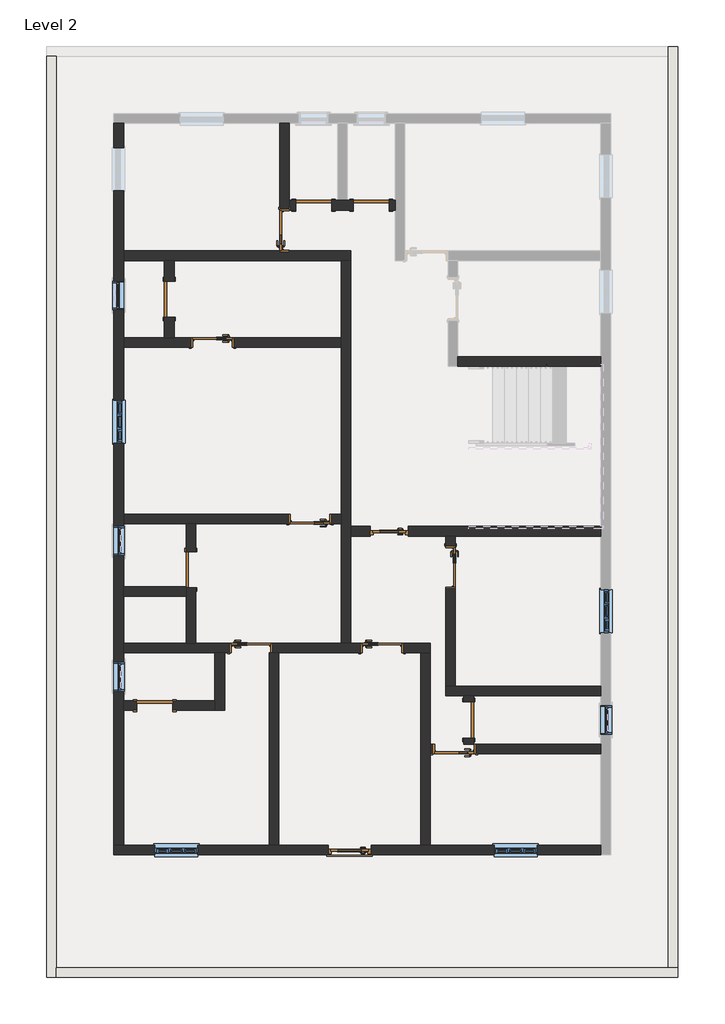
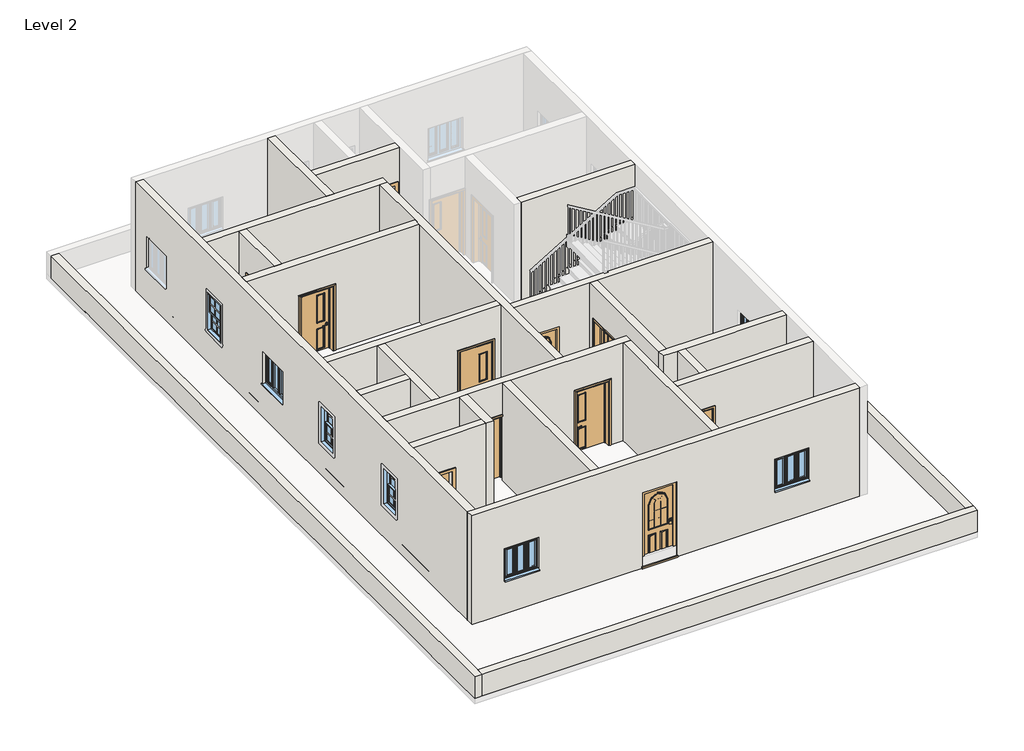
# One storey, part 1 of 3: 25 walls, 15 doors, 8 windows.
"""IFC4 building model written with IfcOpenShell, lengths in millimetres."""

from ifc_helpers import new_model, si_unit, frame, origin, place, context, project, spatial, polyline, outline, extrude, faceted_brep, transform, mapped, element, save
from components import doors_extsgl_w_glazing_bars_arched_810x2110mm_57ea6d9e, doors_extsgl_w_glazing_bars_arched_910x2110mm_1ab485ba, door_aa1d4bf3, door_2f4bc105, door_fadea3f2, door_53b1b562, window_679d2811, windows_tpl_w_glazing_bars_910x910mm_9d987a72

model = new_model("IFC4")

# Units and contexts
model_context = context("Model", 3, world=origin())
ifc_project = project(units=[si_unit("LENGTHUNIT", "METRE", prefix="MILLI")], contexts=[model_context])

# Site, building, storey
site = spatial("IfcSite", under=ifc_project)
building = spatial("IfcBuilding", under=site)
storey = spatial("IfcBuildingStorey", under=building, Name="Level 2", Elevation=3048.0)

# Doors
placement = place(None, origin())
doors_extsgl_w_glazing_bars_arched_810x2110mm_shape = doors_extsgl_w_glazing_bars_arched_810x2110mm_57ea6d9e(model_context)
element("IfcDoor", 1, ObjectType="Doors_ExtSgl_w-Glazing_Bars_Arched : 810x2110mm", at=placement, inside=storey, context=model_context, shape_type="MappedRepresentation", body=[
    mapped(doors_extsgl_w_glazing_bars_arched_810x2110mm_shape, transform((-8090.5711241, 8252.7344295, 3048.0), x_axis=(-1.0, 0.0, 0.0), y_axis=(0.0, -1.0, 0.0), z_axis=(0.0, 0.0, 1.0))),
])
doors_extsgl_w_glazing_bars_arched_910x2110mm_shape = doors_extsgl_w_glazing_bars_arched_910x2110mm_1ab485ba(model_context)
element("IfcDoor", 2, ObjectType="Doors_ExtSgl_w-Glazing_Bars_Arched : 910x2110mm", at=placement, inside=storey, context=model_context, shape_type="MappedRepresentation", body=[
    mapped(doors_extsgl_w_glazing_bars_arched_910x2110mm_shape, transform((-8928.7711241, 1521.7344295, 3048.0), x_axis=(-1.0, 0.0, 0.0), y_axis=(0.0, -1.0, 0.0), z_axis=(0.0, 0.0, 1.0))),
])
door_shape = door_aa1d4bf3(model_context)
element("IfcDoor", 3, ObjectType="Doors_IntSgl_3 : 7'-3\"", at=placement, inside=storey, context=model_context, shape_type="MappedRepresentation", body=[
    mapped(door_shape, transform((-10300.3711241, 14602.7344295, 3048.0), x_axis=(0.0, 1.0, 0.0), y_axis=(-1.0, 0.0, 0.0), z_axis=(0.0, 0.0, 1.0))),
])
element("IfcDoor", 4, ObjectType="Doors_IntSgl_3 : 7'-3\"", at=placement, inside=storey, context=model_context, shape_type="MappedRepresentation", body=[
    mapped(door_shape, transform((-8242.9711241, 5788.9344295, 3048.0), x_axis=(1.0, 0.0, 0.0), y_axis=(0.0, 1.0, 0.0), z_axis=(0.0, 0.0, 1.0))),
])
element("IfcDoor", 5, ObjectType="Doors_IntSgl_3 : 7'-3\"", at=placement, inside=storey, context=model_context, shape_type="MappedRepresentation", body=[
    mapped(door_shape, transform((-6795.1711241, 7490.7344295, 3048.0), x_axis=(0.0, -1.0, 0.0), y_axis=(1.0, 0.0, 0.0), z_axis=(0.0, 0.0, 1.0))),
])
element("IfcDoor", 6, ObjectType="Doors_IntSgl_3 : 7'-3\"", at=placement, inside=storey, context=model_context, shape_type="MappedRepresentation", body=[
    mapped(door_shape, transform((-11011.5711241, 5788.9344295, 3048.0), x_axis=(1.0, 0.0, 0.0), y_axis=(0.0, 1.0, 0.0), z_axis=(0.0, 0.0, 1.0))),
])
element("IfcDoor", 7, ObjectType="Doors_IntSgl_3 : 7'-3\"", at=placement, inside=storey, context=model_context, shape_type="MappedRepresentation", body=[
    mapped(door_shape, transform((-9766.9711241, 8506.7344295, 3048.0), x_axis=(-1.0, 0.0, 0.0), y_axis=(0.0, -1.0, 0.0), z_axis=(0.0, 0.0, 1.0))),
])
element("IfcDoor", 8, ObjectType="Doors_IntSgl_3 : 7'-3\"", at=placement, inside=storey, context=model_context, shape_type="MappedRepresentation", body=[
    mapped(door_shape, transform((-6718.9711241, 3655.3344295, 3048.0), x_axis=(-1.0, 0.0, 0.0), y_axis=(0.0, -1.0, 0.0), z_axis=(0.0, 0.0, 1.0))),
])
door_2_shape = door_2f4bc105(model_context)
element("IfcDoor", 9, ObjectType="Doors_IntSgl_3 : 7'-3\"", at=placement, inside=storey, context=model_context, shape_type="MappedRepresentation", body=[
    mapped(door_2_shape, transform((-11824.3711241, 12240.5344295, 3048.0), x_axis=(-1.0, 0.0, 0.0), y_axis=(0.0, -1.0, 0.0), z_axis=(0.0, 0.0, 1.0))),
])
door_3_shape = door_fadea3f2(model_context)
element("IfcDoor", 10, ObjectType="Single-Flush : 30\" x 80\"", at=placement, inside=storey, context=model_context, shape_type="MappedRepresentation", body=[
    mapped(door_3_shape, transform((-6414.1711241, 4264.9344295, 3048.0), x_axis=(0.0, -1.0, 0.0), y_axis=(1.0, 0.0, 0.0), z_axis=(0.0, 0.0, 1.0))),
])
door_4_shape = door_53b1b562(model_context)
element("IfcDoor", 11, ObjectType="Single-Flush : 30\" x 80\"", at=placement, inside=storey, context=model_context, shape_type="MappedRepresentation", body=[
    mapped(door_4_shape, transform((-13043.5711241, 4569.7344295, 3048.0), x_axis=(-1.0, 0.0, 0.0), y_axis=(0.0, -1.0, 0.0), z_axis=(0.0, 0.0, 1.0))),
])
element("IfcDoor", 12, ObjectType="Single-Flush : 30\" x 80\"", at=placement, inside=storey, context=model_context, shape_type="MappedRepresentation", body=[
    mapped(door_4_shape, transform((-12281.5711241, 7439.9344295, 3048.0), x_axis=(0.0, -1.0, 0.0), y_axis=(1.0, 0.0, 0.0), z_axis=(0.0, 0.0, 1.0))),
])
element("IfcDoor", 13, ObjectType="Single-Flush : 30\" x 80\"", at=placement, inside=storey, context=model_context, shape_type="MappedRepresentation", body=[
    mapped(door_4_shape, transform((-12738.7711241, 13154.9344295, 3048.0), x_axis=(0.0, -1.0, 0.0), y_axis=(1.0, 0.0, 0.0), z_axis=(0.0, 0.0, 1.0))),
])
element("IfcDoor", 14, ObjectType="Single-Flush : 30\" x 80\"", at=placement, inside=storey, context=model_context, shape_type="MappedRepresentation", body=[
    mapped(door_4_shape, transform((-9690.7711241, 15136.1344295, 3048.0), x_axis=(-1.0, 0.0, 0.0), y_axis=(0.0, -1.0, 0.0), z_axis=(0.0, 0.0, 1.0))),
])
element("IfcDoor", 15, ObjectType="Single-Flush : 30\" x 80\"", at=placement, inside=storey, context=model_context, shape_type="MappedRepresentation", body=[
    mapped(door_4_shape, transform((-8471.5711241, 15136.1344295, 3048.0), x_axis=(-1.0, 0.0, 0.0), y_axis=(0.0, -1.0, 0.0), z_axis=(0.0, 0.0, 1.0))),
])

# Walls
element("IfcWall", 16, ObjectType="Generic -4.5\" p", at=placement, inside=storey, context=model_context, shape_type="Brep", body=[
    faceted_brep([(-10401.9711241, 14170.9344295, 6096.0), (-10401.9711241, 16863.3344295, 6096.0), (-10401.9711241, 16863.3344295, 3048.0), (-10401.9711241, 15059.9344295, 3048.0), (-10401.9711241, 15059.9344295, 5181.6), (-10401.9711241, 14170.9344295, 5181.6), (-10198.7711241, 16863.3344295, 6096.0), (-10198.7711241, 15237.7344295, 6096.0), (-10198.7711241, 15034.5344295, 6096.0), (-10198.7711241, 14170.9344295, 6096.0), (-10198.7711241, 14170.9344295, 5181.6), (-10198.7711241, 15059.9344295, 5181.6), (-10198.7711241, 15059.9344295, 3048.0), (-10198.7711241, 15237.7344295, 3048.0), (-10198.7711241, 16863.3344295, 3048.0)], [[[0, 1, 2, 3, 4, 5]], [[6, 7, 8, 9, 10, 11, 12, 13, 14]], [[2, 14, 13, 12, 3]], [[1, 0, 9, 8, 7, 6]], [[2, 1, 6, 14]], [[9, 0, 5, 10]], [[11, 4, 3, 12]], [[4, 11, 10, 5]]]),
])
element("IfcWall", 17, ObjectType="Generic -4.5\" p", at=placement, inside=storey, context=model_context, shape_type="Brep", body=[
    faceted_brep([(-9309.7711241, 15034.5344295, 3048.0), (-8852.5711241, 15034.5344295, 3048.0), (-8852.5711241, 15034.5344295, 5080.0), (-8090.5711241, 15034.5344295, 5080.0), (-8090.5711241, 15034.5344295, 3048.0), (-7963.5711241, 15034.5344295, 3048.0), (-7963.5711241, 15034.5344295, 6096.0), (-10198.7711241, 15034.5344295, 6096.0), (-10198.7711241, 15034.5344295, 3048.0), (-10071.7711241, 15034.5344295, 3048.0), (-10071.7711241, 15034.5344295, 5080.0), (-9309.7711241, 15034.5344295, 5080.0), (-8852.5711241, 15237.7344295, 5080.0), (-8852.5711241, 15237.7344295, 3048.0), (-8979.5711241, 15237.7344295, 3048.0), (-9182.7711241, 15237.7344295, 3048.0), (-9309.7711241, 15237.7344295, 3048.0), (-9309.7711241, 15237.7344295, 5080.0), (-10071.7711241, 15237.7344295, 5080.0), (-10071.7711241, 15237.7344295, 3048.0), (-10198.7711241, 15237.7344295, 3048.0), (-10198.7711241, 15237.7344295, 6096.0), (-9182.7711241, 15237.7344295, 6096.0), (-8979.5711241, 15237.7344295, 6096.0), (-7963.5711241, 15237.7344295, 6096.0), (-7963.5711241, 15237.7344295, 3048.0), (-8090.5711241, 15237.7344295, 3048.0), (-8090.5711241, 15237.7344295, 5080.0), (-10198.7711241, 15059.9344295, 3048.0)], [[[0, 1, 2, 3, 4, 5, 6, 7, 8, 9, 10, 11]], [[12, 13, 14, 15, 16, 17, 18, 19, 20, 21, 22, 23, 24, 25, 26, 27]], [[20, 19, 9, 8, 28]], [[26, 25, 5, 4]], [[16, 15, 14, 13, 1, 0]], [[7, 6, 24, 23, 22, 21]], [[8, 7, 21, 20, 28]], [[6, 5, 25, 24]], [[10, 9, 19, 18]], [[11, 10, 18, 17]], [[0, 11, 17, 16]], [[2, 1, 13, 12]], [[3, 2, 12, 27]], [[4, 3, 27, 26]]]),
])
element("IfcWall", 18, ObjectType="Generic -4.5\" p", at=placement, inside=storey, context=model_context, shape_type="Brep", body=[
    faceted_brep([(-13703.9711241, 13967.7344295, 3048.0), (-12840.3711241, 13967.7344295, 3048.0), (-12637.1711241, 13967.7344295, 3048.0), (-9106.5711241, 13967.7344295, 3048.0), (-8903.3711241, 13967.7344295, 3048.0), (-8903.3711241, 13967.7344295, 6096.0), (-9106.5711241, 13967.7344295, 6096.0), (-12637.1711241, 13967.7344295, 6096.0), (-12840.3711241, 13967.7344295, 6096.0), (-13703.9711241, 13967.7344295, 6096.0), (-13703.9711241, 14170.9344295, 6096.0), (-10401.9711241, 14170.9344295, 6096.0), (-10198.7711241, 14170.9344295, 6096.0), (-8903.3711241, 14170.9344295, 6096.0), (-8903.3711241, 14170.9344295, 3048.0), (-10198.7711241, 14170.9344295, 3048.0), (-10198.7711241, 14170.9344295, 5181.6), (-10401.9711241, 14170.9344295, 5181.6), (-10401.9711241, 14170.9344295, 3048.0), (-13703.9711241, 14170.9344295, 3048.0), (-10401.9711241, 14145.5344295, 3048.0), (-10198.7711241, 14145.5344295, 3048.0), (-10198.7711241, 14145.5344295, 5181.6), (-10401.9711241, 14145.5344295, 5181.6)], [[[0, 1, 2, 3, 4, 5, 6, 7, 8, 9]], [[10, 11, 12, 13, 14, 15, 16, 17, 18, 19]], [[4, 3, 2, 1, 0, 19, 18, 20, 21, 15, 14]], [[9, 8, 7, 6, 5, 13, 12, 11, 10]], [[0, 9, 10, 19]], [[5, 4, 14, 13]], [[21, 22, 16, 15]], [[23, 20, 18, 17]], [[22, 23, 17, 16]], [[22, 21, 20, 23]]]),
])
element("IfcWall", 19, ObjectType="Generic -4.5\" p", at=placement, inside=storey, context=model_context, shape_type="Brep", body=[
    faceted_brep([(-9106.5711241, 13967.7344295, 3048.0), (-9106.5711241, 12342.1344295, 3048.0), (-9106.5711241, 12138.9344295, 3048.0), (-9106.5711241, 8608.3344295, 3048.0), (-9106.5711241, 8405.1344295, 3048.0), (-9106.5711241, 5890.5344295, 3048.0), (-9106.5711241, 5890.5344295, 6096.0), (-9106.5711241, 8405.1344295, 6096.0), (-9106.5711241, 8608.3344295, 6096.0), (-9106.5711241, 12138.9344295, 6096.0), (-9106.5711241, 12342.1344295, 6096.0), (-9106.5711241, 13967.7344295, 6096.0), (-8903.3711241, 13967.7344295, 3048.0), (-8903.3711241, 13967.7344295, 6096.0), (-8903.3711241, 8354.3344295, 6096.0), (-8903.3711241, 8151.1344295, 6096.0), (-8903.3711241, 5890.5344295, 6096.0), (-8903.3711241, 5890.5344295, 3048.0), (-8903.3711241, 8151.1344295, 3048.0), (-8903.3711241, 8354.3344295, 3048.0)], [[[0, 1, 2, 3, 4, 5, 6, 7, 8, 9, 10, 11]], [[12, 13, 14, 15, 16, 17, 18, 19]], [[5, 4, 3, 2, 1, 0, 12, 19, 18, 17]], [[11, 10, 9, 8, 7, 6, 16, 15, 14, 13]], [[0, 11, 13, 12]], [[6, 5, 17, 16]]]),
])
element("IfcWall", 20, ObjectType="Generic -4.5\" p", at=placement, inside=storey, context=model_context, shape_type="Brep", body=[
    faceted_brep([(-13703.9711241, 12342.1344295, 6096.0), (-12840.3711241, 12342.1344295, 6096.0), (-12637.1711241, 12342.1344295, 6096.0), (-9106.5711241, 12342.1344295, 6096.0), (-9106.5711241, 12342.1344295, 3048.0), (-11367.1711241, 12342.1344295, 3048.0), (-11367.1711241, 12342.1344295, 5181.6), (-12281.5711241, 12342.1344295, 5181.6), (-12281.5711241, 12342.1344295, 3048.0), (-12637.1711241, 12342.1344295, 3048.0), (-12840.3711241, 12342.1344295, 3048.0), (-13703.9711241, 12342.1344295, 3048.0), (-9106.5711241, 12138.9344295, 6096.0), (-13703.9711241, 12138.9344295, 6096.0), (-13703.9711241, 12138.9344295, 3048.0), (-12281.5711241, 12138.9344295, 3048.0), (-12281.5711241, 12138.9344295, 5181.6), (-11367.1711241, 12138.9344295, 5181.6), (-11367.1711241, 12138.9344295, 3048.0), (-9106.5711241, 12138.9344295, 3048.0)], [[[0, 1, 2, 3, 4, 5, 6, 7, 8, 9, 10, 11]], [[12, 13, 14, 15, 16, 17, 18, 19]], [[4, 19, 18, 5]], [[14, 11, 10, 9, 8, 15]], [[3, 2, 1, 0, 13, 12]], [[4, 3, 12, 19]], [[0, 11, 14, 13]], [[7, 16, 15, 8]], [[16, 7, 6, 17]], [[17, 6, 5, 18]]]),
])
element("IfcWall", 21, ObjectType="Generic -4.5\" p", at=placement, inside=storey, context=model_context, shape_type="SweptSolid", body=[
    extrude(outline(polyline([(12773.9344295, 5080.0), (12773.9344295, 3048.0), (12342.1344295, 3048.0), (12342.1344295, 6096.0), (13967.7344295, 6096.0), (13967.7344295, 3048.0), (13535.9344295, 3048.0), (13535.9344295, 5080.0), (12773.9344295, 5080.0)])), frame((-12840.3711241, 0.0, 0.0), z_axis=(1.0, 0.0, 0.0), x_axis=(0.0, 1.0, 0.0)), (0.0, 0.0, 1.0), 203.2),
])
element("IfcWall", 22, ObjectType="Generic -4.5\" p", at=placement, inside=storey, context=model_context, shape_type="Brep", body=[
    faceted_brep([(-9106.5711241, 8405.1344295, 6096.0), (-12179.9711241, 8405.1344295, 6096.0), (-12383.1711241, 8405.1344295, 6096.0), (-13703.9711241, 8405.1344295, 6096.0), (-13703.9711241, 8405.1344295, 3048.0), (-12383.1711241, 8405.1344295, 3048.0), (-12179.9711241, 8405.1344295, 3048.0), (-10224.1711241, 8405.1344295, 3048.0), (-10224.1711241, 8405.1344295, 5181.6), (-9309.7711241, 8405.1344295, 5181.6), (-9309.7711241, 8405.1344295, 3048.0), (-9106.5711241, 8405.1344295, 3048.0), (-13703.9711241, 8608.3344295, 6096.0), (-9106.5711241, 8608.3344295, 6096.0), (-9106.5711241, 8608.3344295, 3048.0), (-9309.7711241, 8608.3344295, 3048.0), (-9309.7711241, 8608.3344295, 5181.6), (-10224.1711241, 8608.3344295, 5181.6), (-10224.1711241, 8608.3344295, 3048.0), (-13703.9711241, 8608.3344295, 3048.0)], [[[0, 1, 2, 3, 4, 5, 6, 7, 8, 9, 10, 11]], [[12, 13, 14, 15, 16, 17, 18, 19]], [[4, 19, 18, 7, 6, 5]], [[14, 11, 10, 15]], [[3, 2, 1, 0, 13, 12]], [[4, 3, 12, 19]], [[0, 11, 14, 13]], [[17, 8, 7, 18]], [[8, 17, 16, 9]], [[9, 16, 15, 10]]]),
])
element("IfcWall", 23, ObjectType="Generic -4.5\" p", at=placement, inside=storey, context=model_context, shape_type="Brep", body=[
    faceted_brep([(-12383.1711241, 7058.9344295, 5080.0), (-12383.1711241, 7058.9344295, 3048.0), (-12383.1711241, 6881.1344295, 3048.0), (-12383.1711241, 5890.5344295, 3048.0), (-12383.1711241, 5890.5344295, 6096.0), (-12383.1711241, 6881.1344295, 6096.0), (-12383.1711241, 7084.3344295, 6096.0), (-12383.1711241, 8405.1344295, 6096.0), (-12383.1711241, 8405.1344295, 3048.0), (-12383.1711241, 7820.9344295, 3048.0), (-12383.1711241, 7820.9344295, 5080.0), (-12179.9711241, 5890.5344295, 3048.0), (-12179.9711241, 7058.9344295, 3048.0), (-12179.9711241, 7058.9344295, 5080.0), (-12179.9711241, 7820.9344295, 5080.0), (-12179.9711241, 7820.9344295, 3048.0), (-12179.9711241, 8405.1344295, 3048.0), (-12179.9711241, 8405.1344295, 6096.0), (-12179.9711241, 5890.5344295, 6096.0)], [[[0, 1, 2, 3, 4, 5, 6, 7, 8, 9, 10]], [[11, 12, 13, 14, 15, 16, 17, 18]], [[9, 8, 16, 15]], [[3, 2, 1, 12, 11]], [[7, 6, 5, 4, 18, 17]], [[8, 7, 17, 16]], [[4, 3, 11, 18]], [[13, 12, 1, 0]], [[14, 13, 0, 10]], [[15, 14, 10, 9]]]),
])
element("IfcWall", 24, ObjectType="Generic -4.5\" p", at=placement, inside=storey, context=model_context, shape_type="Brep", body=[
    faceted_brep([(-13703.9711241, 6881.1344295, 3048.0), (-12383.1711241, 6881.1344295, 3048.0), (-12383.1711241, 6881.1344295, 6096.0), (-13703.9711241, 6881.1344295, 6096.0), (-13703.9711241, 7084.3344295, 3048.0), (-13703.9711241, 7084.3344295, 6096.0), (-12383.1711241, 7084.3344295, 6096.0), (-12383.1711241, 7084.3344295, 3048.0), (-12383.1711241, 7058.9344295, 3048.0)], [[[0, 1, 2, 3]], [[4, 5, 6, 7]], [[1, 0, 4, 7, 8]], [[3, 2, 6, 5]], [[0, 3, 5, 4]], [[2, 1, 8, 7, 6]]]),
])
element("IfcWall", 25, ObjectType="Generic -4.5\" p", at=placement, inside=storey, context=model_context, shape_type="Brep", body=[
    faceted_brep([(-7226.9711241, 5687.3344295, 6096.0), (-7430.1711241, 5687.3344295, 6096.0), (-10427.3711241, 5687.3344295, 6096.0), (-10630.5711241, 5687.3344295, 6096.0), (-11570.3711241, 5687.3344295, 6096.0), (-11773.5711241, 5687.3344295, 6096.0), (-13703.9711241, 5687.3344295, 6096.0), (-13703.9711241, 5687.3344295, 3048.0), (-11773.5711241, 5687.3344295, 3048.0), (-11570.3711241, 5687.3344295, 3048.0), (-11468.7711241, 5687.3344295, 3048.0), (-11468.7711241, 5687.3344295, 5181.6), (-10554.3711241, 5687.3344295, 5181.6), (-10554.3711241, 5687.3344295, 3048.0), (-10427.3711241, 5687.3344295, 3048.0), (-8700.1711241, 5687.3344295, 3048.0), (-8700.1711241, 5687.3344295, 5181.6), (-7785.7711241, 5687.3344295, 5181.6), (-7785.7711241, 5687.3344295, 3048.0), (-7430.1711241, 5687.3344295, 3048.0), (-7226.9711241, 5687.3344295, 3048.0), (-13703.9711241, 5890.5344295, 6096.0), (-12383.1711241, 5890.5344295, 6096.0), (-12179.9711241, 5890.5344295, 6096.0), (-9106.5711241, 5890.5344295, 6096.0), (-8903.3711241, 5890.5344295, 6096.0), (-7226.9711241, 5890.5344295, 6096.0), (-7226.9711241, 5890.5344295, 3048.0), (-7785.7711241, 5890.5344295, 3048.0), (-7785.7711241, 5890.5344295, 5181.6), (-8700.1711241, 5890.5344295, 5181.6), (-8700.1711241, 5890.5344295, 3048.0), (-8903.3711241, 5890.5344295, 3048.0), (-9106.5711241, 5890.5344295, 3048.0), (-10554.3711241, 5890.5344295, 3048.0), (-10554.3711241, 5890.5344295, 5181.6), (-11468.7711241, 5890.5344295, 5181.6), (-11468.7711241, 5890.5344295, 3048.0), (-12179.9711241, 5890.5344295, 3048.0), (-12383.1711241, 5890.5344295, 3048.0), (-13703.9711241, 5890.5344295, 3048.0)], [[[0, 1, 2, 3, 4, 5, 6, 7, 8, 9, 10, 11, 12, 13, 14, 15, 16, 17, 18, 19, 20]], [[21, 22, 23, 24, 25, 26, 27, 28, 29, 30, 31, 32, 33, 34, 35, 36, 37, 38, 39, 40]], [[7, 40, 39, 38, 37, 10, 9, 8]], [[27, 20, 19, 18, 28]], [[31, 15, 14, 13, 34, 33, 32]], [[6, 5, 4, 3, 2, 1, 0, 26, 25, 24, 23, 22, 21]], [[7, 6, 21, 40]], [[0, 20, 27, 26]], [[17, 29, 28, 18]], [[29, 17, 16, 30]], [[30, 16, 15, 31]], [[12, 35, 34, 13]], [[35, 12, 11, 36]], [[36, 11, 10, 37]]]),
])
element("IfcWall", 26, ObjectType="Generic -4.5\" p", at=placement, inside=storey, context=model_context, shape_type="Brep", body=[
    faceted_brep([(-7430.1711241, 5687.3344295, 3048.0), (-7430.1711241, 1623.3344295, 3048.0), (-7430.1711241, 1623.3344295, 6096.0), (-7430.1711241, 5687.3344295, 6096.0), (-7226.9711241, 5687.3344295, 3048.0), (-7226.9711241, 5687.3344295, 6096.0), (-7226.9711241, 3756.9344295, 6096.0), (-7226.9711241, 3553.7344295, 6096.0), (-7226.9711241, 1623.3344295, 6096.0), (-7226.9711241, 1623.3344295, 3048.0), (-7226.9711241, 3553.7344295, 3048.0), (-7226.9711241, 3756.9344295, 3048.0)], [[[0, 1, 2, 3]], [[4, 5, 6, 7, 8, 9, 10, 11]], [[1, 0, 4, 11, 10, 9]], [[3, 2, 8, 7, 6, 5]], [[0, 3, 5, 4]], [[2, 1, 9, 8]]]),
])
element("IfcWall", 27, ObjectType="Generic -4.5\" p", at=placement, inside=storey, context=model_context, shape_type="Brep", body=[
    faceted_brep([(-11773.5711241, 5687.3344295, 3048.0), (-11773.5711241, 4671.3344295, 3048.0), (-11773.5711241, 4468.1344295, 3048.0), (-11773.5711241, 4468.1344295, 6096.0), (-11773.5711241, 4671.3344295, 6096.0), (-11773.5711241, 5687.3344295, 6096.0), (-11570.3711241, 5687.3344295, 3048.0), (-11570.3711241, 5687.3344295, 6096.0), (-11570.3711241, 4468.1344295, 6096.0), (-11570.3711241, 4468.1344295, 3048.0)], [[[0, 1, 2, 3, 4, 5]], [[6, 7, 8, 9]], [[2, 1, 0, 6, 9]], [[5, 4, 3, 8, 7]], [[0, 5, 7, 6]], [[3, 2, 9, 8]]]),
])
element("IfcWall", 28, ObjectType="Generic -4.5\" p", at=placement, inside=storey, context=model_context, shape_type="SweptSolid", body=[
    extrude(outline(polyline([(3048.0, -13703.9711241), (3048.0, -13424.5711241), (5080.0, -13424.5711241), (5080.0, -12662.5711241), (3048.0, -12662.5711241), (3048.0, -11773.5711241), (6096.0, -11773.5711241), (6096.0, -13703.9711241), (3048.0, -13703.9711241)])), frame((0.0, 4468.1344295, 0.0), z_axis=(0.0, 1.0, 0.0), x_axis=(0.0, 0.0, 1.0)), (0.0, 0.0, 1.0), 203.2),
])
element("IfcWall", 29, ObjectType="Generic -4.5\" p", at=placement, inside=storey, context=model_context, shape_type="Brep", body=[
    faceted_brep([(-10630.5711241, 5687.3344295, 3048.0), (-10630.5711241, 1623.3344295, 3048.0), (-10630.5711241, 1623.3344295, 6096.0), (-10630.5711241, 5687.3344295, 6096.0), (-10427.3711241, 5687.3344295, 3048.0), (-10427.3711241, 5687.3344295, 6096.0), (-10427.3711241, 1623.3344295, 6096.0), (-10427.3711241, 1623.3344295, 3048.0), (-10554.3711241, 5687.3344295, 3048.0)], [[[0, 1, 2, 3]], [[4, 5, 6, 7]], [[1, 0, 8, 4, 7]], [[3, 2, 6, 5]], [[2, 1, 7, 6]], [[0, 3, 5, 4, 8]]]),
])
element("IfcWall", 30, ObjectType="Generic -4.5\" p", at=placement, inside=storey, context=model_context, shape_type="Brep", body=[
    faceted_brep([(-3620.1711241, 3553.7344295, 6096.0), (-7226.9711241, 3553.7344295, 6096.0), (-7226.9711241, 3553.7344295, 3048.0), (-7176.1711241, 3553.7344295, 3048.0), (-7176.1711241, 3553.7344295, 5181.6), (-6261.7711241, 3553.7344295, 5181.6), (-6261.7711241, 3553.7344295, 3048.0), (-3620.1711241, 3553.7344295, 3048.0), (-7226.9711241, 3756.9344295, 6096.0), (-6515.7711241, 3756.9344295, 6096.0), (-6312.5711241, 3756.9344295, 6096.0), (-3620.1711241, 3756.9344295, 6096.0), (-3620.1711241, 3756.9344295, 3048.0), (-6261.7711241, 3756.9344295, 3048.0), (-6261.7711241, 3756.9344295, 5181.6), (-7176.1711241, 3756.9344295, 5181.6), (-7176.1711241, 3756.9344295, 3048.0), (-7226.9711241, 3756.9344295, 3048.0)], [[[0, 1, 2, 3, 4, 5, 6, 7]], [[8, 9, 10, 11, 12, 13, 14, 15, 16, 17]], [[2, 17, 16, 3]], [[12, 7, 6, 13]], [[1, 0, 11, 10, 9, 8]], [[0, 7, 12, 11]], [[2, 1, 8, 17]], [[15, 4, 3, 16]], [[4, 15, 14, 5]], [[5, 14, 13, 6]]]),
])
element("IfcWall", 31, ObjectType="Generic -4.5\" p", at=placement, inside=storey, context=model_context, shape_type="SweptSolid", body=[
    extrude(outline(polyline([(3883.9344295, 5080.0), (3883.9344295, 3048.0), (3756.9344295, 3048.0), (3756.9344295, 6096.0), (4772.9344295, 6096.0), (4772.9344295, 3048.0), (4645.9344295, 3048.0), (4645.9344295, 5080.0), (3883.9344295, 5080.0)])), frame((-6515.7711241, 0.0, 0.0), z_axis=(1.0, 0.0, 0.0), x_axis=(0.0, 1.0, 0.0)), (0.0, 0.0, 1.0), 203.2),
])
element("IfcWall", 32, ObjectType="Generic -4.5\" p", at=placement, inside=storey, context=model_context, shape_type="Brep", body=[
    faceted_brep([(-3620.1711241, 4976.1344295, 3048.0), (-6693.5711241, 4976.1344295, 3048.0), (-6896.7711241, 4976.1344295, 3048.0), (-6896.7711241, 4976.1344295, 6096.0), (-6693.5711241, 4976.1344295, 6096.0), (-3620.1711241, 4976.1344295, 6096.0), (-3620.1711241, 4772.9344295, 3048.0), (-3620.1711241, 4772.9344295, 6096.0), (-6312.5711241, 4772.9344295, 6096.0), (-6515.7711241, 4772.9344295, 6096.0), (-6896.7711241, 4772.9344295, 6096.0), (-6896.7711241, 4772.9344295, 3048.0), (-6515.7711241, 4772.9344295, 3048.0), (-6312.5711241, 4772.9344295, 3048.0)], [[[0, 1, 2, 3, 4, 5]], [[6, 7, 8, 9, 10, 11, 12, 13]], [[2, 1, 0, 6, 13, 12, 11]], [[5, 4, 3, 10, 9, 8, 7]], [[0, 5, 7, 6]], [[3, 2, 11, 10]]]),
])
element("IfcWall", 33, ObjectType="Generic -4.5\" p", at=placement, inside=storey, context=model_context, shape_type="SweptSolid", body=[
    extrude(outline(polyline([(4976.1344295, 6096.0), (8151.1344295, 6096.0), (8151.1344295, 3048.0), (7947.9344295, 3048.0), (7947.9344295, 5181.6), (7033.5344295, 5181.6), (7033.5344295, 3048.0), (4976.1344295, 3048.0), (4976.1344295, 6096.0)])), frame((-6896.7711241, 0.0, 0.0), z_axis=(1.0, 0.0, 0.0), x_axis=(0.0, 1.0, 0.0)), (0.0, 0.0, 1.0), 203.2),
])
element("IfcWall", 34, ObjectType="Generic -4.5\" p", at=placement, inside=storey, context=model_context, shape_type="SweptSolid", body=[
    extrude(outline(polyline([(-3620.1711241, 11732.5344295), (-6642.7711241, 11732.5344295), (-6642.7711241, 11935.7344295), (-3620.1711241, 11935.7344295), (-3620.1711241, 11732.5344295)])), frame((0.0, 0.0, 3048.0), z_axis=(0.0, 0.0, 1.0), x_axis=(1.0, 0.0, 0.0)), (0.0, 0.0, 1.0), 3048.0),
])
element("IfcWall", 35, ObjectType="Generic -4.5\" p", at=placement, inside=storey, context=model_context, shape_type="Brep", body=[
    faceted_brep([(-8495.5711241, 8354.3344295, 5158.0), (-8495.5711241, 8354.3344295, 3048.0), (-8903.3711241, 8354.3344295, 3048.0), (-8903.3711241, 8354.3344295, 6096.0), (-3620.1711241, 8354.3344295, 6096.0), (-3620.1711241, 8354.3344295, 3048.0), (-7685.5711241, 8354.3344295, 3048.0), (-7685.5711241, 8354.3344295, 5158.0), (-8903.3711241, 8151.1344295, 3048.0), (-8495.5711241, 8151.1344295, 3048.0), (-8495.5711241, 8151.1344295, 5158.0), (-7685.5711241, 8151.1344295, 5158.0), (-7685.5711241, 8151.1344295, 3048.0), (-6896.7711241, 8151.1344295, 3048.0), (-6693.5711241, 8151.1344295, 3048.0), (-3620.1711241, 8151.1344295, 3048.0), (-3620.1711241, 8151.1344295, 6096.0), (-6693.5711241, 8151.1344295, 6096.0), (-6896.7711241, 8151.1344295, 6096.0), (-8903.3711241, 8151.1344295, 6096.0)], [[[0, 1, 2, 3, 4, 5, 6, 7]], [[8, 9, 10, 11, 12, 13, 14, 15, 16, 17, 18, 19]], [[6, 5, 15, 14, 13, 12]], [[2, 1, 9, 8]], [[4, 3, 19, 18, 17, 16]], [[5, 4, 16, 15]], [[3, 2, 8, 19]], [[12, 11, 7, 6]], [[10, 9, 1, 0]], [[11, 10, 0, 7]]]),
])
element("IfcWall", 36, ObjectType="Generic -4.5\" p", at=placement, inside=storey, context=model_context, shape_type="Brep", body=[
    faceted_brep([(-15126.3711241, -1171.3990222, 3048.0), (-15126.3711241, -968.1990222, 3048.0), (-15126.3711241, 18285.0009778, 3048.0), (-15126.3711241, 18285.0009778, 3657.6), (-15126.3711241, -968.1990222, 3657.6), (-15126.3711241, -1171.3990222, 3657.6), (-15329.5711241, -1171.3990222, 3048.0), (-15329.5711241, -1171.3990222, 3657.6), (-15329.5711241, 18285.0009778, 3657.6), (-15329.5711241, 18285.0009778, 3048.0)], [[[0, 1, 2, 3, 4, 5]], [[6, 7, 8, 9]], [[2, 1, 0, 6, 9]], [[5, 4, 3, 8, 7]], [[0, 5, 7, 6]], [[3, 2, 9, 8]]]),
])
element("IfcWall", 37, ObjectType="Generic -4.5\" p", at=placement, inside=storey, context=model_context, shape_type="Brep", body=[
    faceted_brep([(-1994.5711241, -968.1990222, 3048.0), (-2197.7711241, -968.1990222, 3048.0), (-15126.3711241, -968.1990222, 3048.0), (-15126.3711241, -968.1990222, 3657.6), (-2197.7711241, -968.1990222, 3657.6), (-1994.5711241, -968.1990222, 3657.6), (-1994.5711241, -1171.3990222, 3048.0), (-1994.5711241, -1171.3990222, 3657.6), (-15126.3711241, -1171.3990222, 3657.6), (-15126.3711241, -1171.3990222, 3048.0)], [[[0, 1, 2, 3, 4, 5]], [[6, 7, 8, 9]], [[2, 1, 0, 6, 9]], [[5, 4, 3, 8, 7]], [[0, 5, 7, 6]], [[3, 2, 9, 8]]]),
])
element("IfcWall", 38, ObjectType="Generic -4.5\" p", at=placement, inside=storey, context=model_context, shape_type="Brep", body=[
    faceted_brep([(-2197.7711241, 18488.2009778, 3048.0), (-2197.7711241, 18285.0009778, 3048.0), (-2197.7711241, -968.1990222, 3048.0), (-2197.7711241, -968.1990222, 3657.6), (-2197.7711241, 18285.0009778, 3657.6), (-2197.7711241, 18488.2009778, 3657.6), (-1994.5711241, 18488.2009778, 3048.0), (-1994.5711241, 18488.2009778, 3657.6), (-1994.5711241, -968.1990222, 3657.6), (-1994.5711241, -968.1990222, 3048.0)], [[[0, 1, 2, 3, 4, 5]], [[6, 7, 8, 9]], [[2, 1, 0, 6, 9]], [[5, 4, 3, 8, 7]], [[0, 5, 7, 6]], [[3, 2, 9, 8]]]),
])
element("IfcWall", 39, ObjectType="Generic -9\" w", at=placement, inside=storey, context=model_context, shape_type="Brep", body=[
    faceted_brep([(-9383.7711241, 1623.3344295, 5158.0), (-9383.7711241, 1623.3344295, 3048.0), (-10427.3711241, 1623.3344295, 3048.0), (-10630.5711241, 1623.3344295, 3048.0), (-13703.9711241, 1623.3344295, 3048.0), (-13907.1711241, 1623.3344295, 3048.0), (-13907.1711241, 1623.3344295, 6096.0), (-13703.9711241, 1623.3344295, 6096.0), (-10630.5711241, 1623.3344295, 6096.0), (-10427.3711241, 1623.3344295, 6096.0), (-7430.1711241, 1623.3344295, 6096.0), (-7226.9711241, 1623.3344295, 6096.0), (-3620.1711241, 1623.3344295, 6096.0), (-3620.1711241, 1623.3344295, 3048.0), (-7226.9711241, 1623.3344295, 3048.0), (-7430.1711241, 1623.3344295, 3048.0), (-8473.7711241, 1623.3344295, 3048.0), (-8473.7711241, 1623.3344295, 5158.0), (-12131.3711241, 1623.3344295, 4872.4), (-13041.3711241, 1623.3344295, 4872.4), (-13041.3711241, 1623.3344295, 3962.4), (-12131.3711241, 1623.3344295, 3962.4), (-4968.5711241, 1623.3344295, 4872.4), (-5878.5711241, 1623.3344295, 4872.4), (-5878.5711241, 1623.3344295, 3962.4), (-4968.5711241, 1623.3344295, 3962.4), (-13907.1711241, 1420.1344295, 3048.0), (-9383.7711241, 1420.1344295, 3048.0), (-9383.7711241, 1420.1344295, 5158.0), (-8473.7711241, 1420.1344295, 5158.0), (-8473.7711241, 1420.1344295, 3048.0), (-3620.1711241, 1420.1344295, 3048.0), (-3620.1711241, 1420.1344295, 6096.0), (-13907.1711241, 1420.1344295, 6096.0), (-12131.3711241, 1420.1344295, 4872.4), (-12131.3711241, 1420.1344295, 3962.4), (-13041.3711241, 1420.1344295, 3962.4), (-13041.3711241, 1420.1344295, 4872.4), (-4968.5711241, 1420.1344295, 4872.4), (-4968.5711241, 1420.1344295, 3962.4), (-5878.5711241, 1420.1344295, 3962.4), (-5878.5711241, 1420.1344295, 4872.4)], [[[0, 1, 2, 3, 4, 5, 6, 7, 8, 9, 10, 11, 12, 13, 14, 15, 16, 17], [18, 19, 20, 21], [22, 23, 24, 25]], [[26, 27, 28, 29, 30, 31, 32, 33], [34, 35, 36, 37], [38, 39, 40, 41]], [[5, 4, 3, 2, 1, 27, 26]], [[16, 15, 14, 13, 31, 30]], [[12, 11, 10, 9, 8, 7, 6, 33, 32]], [[13, 12, 32, 31]], [[6, 5, 26, 33]], [[30, 29, 17, 16]], [[28, 27, 1, 0]], [[29, 28, 0, 17]], [[35, 34, 18, 21]], [[36, 35, 21, 20]], [[37, 36, 20, 19]], [[34, 37, 19, 18]], [[39, 38, 22, 25]], [[40, 39, 25, 24]], [[41, 40, 24, 23]], [[38, 41, 23, 22]]]),
])
element("IfcWall", 40, ObjectType="Generic -9\" w", at=placement, inside=storey, context=model_context, shape_type="Brep", body=[
    faceted_brep([(-13703.9711241, 1623.3344295, 3048.0), (-13703.9711241, 4468.1344295, 3048.0), (-13703.9711241, 4671.3344295, 3048.0), (-13703.9711241, 5687.3344295, 3048.0), (-13703.9711241, 5890.5344295, 3048.0), (-13703.9711241, 6881.1344295, 3048.0), (-13703.9711241, 7084.3344295, 3048.0), (-13703.9711241, 8405.1344295, 3048.0), (-13703.9711241, 8608.3344295, 3048.0), (-13703.9711241, 12138.9344295, 3048.0), (-13703.9711241, 12342.1344295, 3048.0), (-13703.9711241, 13967.7344295, 3048.0), (-13703.9711241, 14170.9344295, 3048.0), (-13703.9711241, 16863.3344295, 3048.0), (-13703.9711241, 16863.3344295, 6096.0), (-13703.9711241, 14170.9344295, 6096.0), (-13703.9711241, 13967.7344295, 6096.0), (-13703.9711241, 12342.1344295, 6096.0), (-13703.9711241, 12138.9344295, 6096.0), (-13703.9711241, 8608.3344295, 6096.0), (-13703.9711241, 8405.1344295, 6096.0), (-13703.9711241, 7084.3344295, 6096.0), (-13703.9711241, 6881.1344295, 6096.0), (-13703.9711241, 5890.5344295, 6096.0), (-13703.9711241, 5687.3344295, 6096.0), (-13703.9711241, 4671.3344295, 6096.0), (-13703.9711241, 4468.1344295, 6096.0), (-13703.9711241, 1623.3344295, 6096.0), (-13703.9711241, 11019.1344295, 4872.4), (-13703.9711241, 11019.1344295, 3962.4), (-13703.9711241, 10109.1344295, 3962.4), (-13703.9711241, 10109.1344295, 4872.4), (-13703.9711241, 15443.1344295, 4872.4), (-13703.9711241, 16353.1344295, 4872.4), (-13703.9711241, 16353.1344295, 3962.4), (-13703.9711241, 15443.1344295, 3962.4), (-13703.9711241, 8354.3344295, 5029.2), (-13703.9711241, 8354.3344295, 3962.4), (-13703.9711241, 7744.7344295, 3962.4), (-13703.9711241, 7744.7344295, 5029.2), (-13703.9711241, 5484.1344295, 5029.2), (-13703.9711241, 5484.1344295, 3962.4), (-13703.9711241, 4874.5344295, 3962.4), (-13703.9711241, 4874.5344295, 5029.2), (-13703.9711241, 12926.3344295, 5029.2), (-13703.9711241, 13535.9344295, 5029.2), (-13703.9711241, 13535.9344295, 3962.4), (-13703.9711241, 12926.3344295, 3962.4), (-13907.1711241, 1623.3344295, 3048.0), (-13907.1711241, 1623.3344295, 6096.0), (-13907.1711241, 16863.3344295, 6096.0), (-13907.1711241, 16863.3344295, 3048.0), (-13907.1711241, 11019.1344295, 4872.4), (-13907.1711241, 10109.1344295, 4872.4), (-13907.1711241, 10109.1344295, 3962.4), (-13907.1711241, 11019.1344295, 3962.4), (-13907.1711241, 15443.1344295, 4872.4), (-13907.1711241, 15443.1344295, 3962.4), (-13907.1711241, 16353.1344295, 3962.4), (-13907.1711241, 16353.1344295, 4872.4), (-13907.1711241, 8354.3344295, 5029.2), (-13907.1711241, 7744.7344295, 5029.2), (-13907.1711241, 7744.7344295, 3962.4), (-13907.1711241, 8354.3344295, 3962.4), (-13907.1711241, 5484.1344295, 5029.2), (-13907.1711241, 4874.5344295, 5029.2), (-13907.1711241, 4874.5344295, 3962.4), (-13907.1711241, 5484.1344295, 3962.4), (-13907.1711241, 12926.3344295, 5029.2), (-13907.1711241, 12926.3344295, 3962.4), (-13907.1711241, 13535.9344295, 3962.4), (-13907.1711241, 13535.9344295, 5029.2)], [[[0, 1, 2, 3, 4, 5, 6, 7, 8, 9, 10, 11, 12, 13, 14, 15, 16, 17, 18, 19, 20, 21, 22, 23, 24, 25, 26, 27], [28, 29, 30, 31], [32, 33, 34, 35], [36, 37, 38, 39], [40, 41, 42, 43], [44, 45, 46, 47]], [[48, 49, 50, 51], [52, 53, 54, 55], [56, 57, 58, 59], [60, 61, 62, 63], [64, 65, 66, 67], [68, 69, 70, 71]], [[13, 12, 11, 10, 9, 8, 7, 6, 5, 4, 3, 2, 1, 0, 48, 51]], [[27, 26, 25, 24, 23, 22, 21, 20, 19, 18, 17, 16, 15, 14, 50, 49]], [[0, 27, 49, 48]], [[14, 13, 51, 50]], [[29, 28, 52, 55]], [[30, 29, 55, 54]], [[31, 30, 54, 53]], [[28, 31, 53, 52]], [[57, 56, 32, 35]], [[58, 57, 35, 34]], [[59, 58, 34, 33]], [[56, 59, 33, 32]], [[37, 36, 60, 63]], [[38, 37, 63, 62]], [[39, 38, 62, 61]], [[36, 39, 61, 60]], [[41, 40, 64, 67]], [[42, 41, 67, 66]], [[43, 42, 66, 65]], [[40, 43, 65, 64]], [[69, 68, 44, 47]], [[70, 69, 47, 46]], [[71, 70, 46, 45]], [[68, 71, 45, 44]]]),
])

# Windows
window_shape = window_679d2811(model_context)
element("IfcWindow", 41, ObjectType="Window-Double-Hung : 24\" x 42\"", at=placement, inside=storey, context=model_context, shape_type="MappedRepresentation", body=[
    mapped(window_shape, transform((-13805.5711241, 8049.5344295, 3048.0), x_axis=(0.0, -1.0, 0.0), y_axis=(1.0, 0.0, 0.0), z_axis=(0.0, 0.0, 1.0))),
])
element("IfcWindow", 42, ObjectType="Window-Double-Hung : 24\" x 42\"", at=placement, inside=storey, context=model_context, shape_type="MappedRepresentation", body=[
    mapped(window_shape, transform((-13805.5711241, 5179.3344295, 3048.0), x_axis=(0.0, -1.0, 0.0), y_axis=(1.0, 0.0, 0.0), z_axis=(0.0, 0.0, 1.0))),
])
element("IfcWindow", 43, ObjectType="Window-Double-Hung : 24\" x 42\"", at=placement, inside=storey, context=model_context, shape_type="MappedRepresentation", body=[
    mapped(window_shape, transform((-13805.5711241, 13231.1344295, 3048.0), x_axis=(0.0, 1.0, 0.0), y_axis=(-1.0, 0.0, 0.0), z_axis=(0.0, 0.0, 1.0))),
])
element("IfcWindow", 44, ObjectType="Window-Double-Hung : 24\" x 42\"", at=placement, inside=storey, context=model_context, shape_type="MappedRepresentation", body=[
    mapped(window_shape, transform((-3518.5711241, 4264.9344295, 3048.0), x_axis=(0.0, -1.0, 0.0), y_axis=(1.0, 0.0, 0.0), z_axis=(0.0, 0.0, 1.0))),
])
windows_tpl_w_glazing_bars_910x910mm_shape = windows_tpl_w_glazing_bars_910x910mm_9d987a72(model_context)
element("IfcWindow", 45, ObjectType="Windows_Tpl_w-Glazing_Bars : 910x910mm", at=placement, inside=storey, context=model_context, shape_type="MappedRepresentation", body=[
    mapped(windows_tpl_w_glazing_bars_910x910mm_shape, transform((-12823.0377907, 1530.1909974, 2762.4), x_axis=(-1.0, 0.0, 0.0), y_axis=(0.0, -1.0, 0.0), z_axis=(0.0, 0.0, 1.0))),
])
element("IfcWindow", 46, ObjectType="Windows_Tpl_w-Glazing_Bars : 910x910mm", at=placement, inside=storey, context=model_context, shape_type="MappedRepresentation", body=[
    mapped(windows_tpl_w_glazing_bars_910x910mm_shape, transform((-5660.2377907, 1530.1909974, 2762.4), x_axis=(-1.0, 0.0, 0.0), y_axis=(0.0, -1.0, 0.0), z_axis=(0.0, 0.0, 1.0))),
])
element("IfcWindow", 47, ObjectType="Windows_Tpl_w-Glazing_Bars : 910x910mm", at=placement, inside=storey, context=model_context, shape_type="MappedRepresentation", body=[
    mapped(windows_tpl_w_glazing_bars_910x910mm_shape, transform((-13814.0276919, 10327.4677629, 2762.4), x_axis=(0.0, -1.0, 0.0), y_axis=(1.0, 0.0, 0.0), z_axis=(0.0, 0.0, 1.0))),
])
element("IfcWindow", 48, ObjectType="Windows_Tpl_w-Glazing_Bars : 910x910mm", at=placement, inside=storey, context=model_context, shape_type="MappedRepresentation", body=[
    mapped(windows_tpl_w_glazing_bars_910x910mm_shape, transform((-3527.0276919, 6326.9677629, 2762.4), x_axis=(0.0, -1.0, 0.0), y_axis=(1.0, 0.0, 0.0), z_axis=(0.0, 0.0, 1.0))),
])

save(model, "model.ifc")

# Revit data of these elements
# Type "Doors_ExtSgl_w-Glazing_Bars_Arched : 810x2110mm"
#   Type Mark = "9"
#   Type Comments = "External Single"
#   Operation = "SingleSwingRight"
#   Construction Type Id = "SGL"
#   Keynote = "L20"
#   Analytic Construction = "Large single-glazed windows"
#   Wrap Layers (Int) from Ext = 0' - 6.98819"
#   Wrap Layers (Ext) from Ext = 0' - 4.03543"
#   Visual Light Transmittance = 0.9
#   Thickness = 0' - 1.73228"
#   Solar Heat Gain Coefficient = 0.86
#   Rough Width = 2' - 7.88976"
#   Rough Height = 6' - 11.07087"
#   O/A Frame Width = 0' - 2.51969"
#   Heat Transfer Coefficient (U) = 0.979472 BTU/(h·ft²·°F)
#   Handle Z Distance = 3' - 5.33858"
#   Glazing Thickness = 0' - 0.94488"
#   FrameWidth = 0' - 1.65354"
#   FrameOffset - External = 0' - 0.98425"
#   FrameDepth = 0' - 3.50394"
#   Door Panel Width = 2' - 3.83465"
#   Door Panel Thickness = 0' - 1.73228"
#   Door Panel Height = 6' - 6.74016"
#   DONT CHANGE - Half Glazed Width = 0' - 8.01181"
#   DONT CHANGE - Glazed Width = 1' - 4.02362"
#   Cill Thickness = 0' - 2.14567"
#   Cill Projection = 0' - 1.1811"
#   Handle X Distance = 0' - 2.95276"
#   Height = 6' - 11.07087"
#   Structural Tolerance = 0' - 0.25591"
#   Tolerance = 0' - 0.11811"
#   Undercut = 0' - 0.15748"
#   Width = 2' - 7.88976"
#   Cill Extension = 0' - 0.98425"
#   Cavity Closer Width = 0' - 1.9685"
#   Cavity Closer Offset from Ext = 0' - 4.03543"
#   Cavity Closer Depth = 0' - 3.34646"
#   Vis - Ironmongery = yes
#   Vis - Glazing Bars = yes
#   Vis - Cavity Closers = yes
#   Define Thermal Properties by = 1
#   Function = 1
#   Material Glass = Door - Glazing
#   Material Glazing Bar = Door - Panel
#   Material Door = Door - Panel
#   Material Frame = Door - Frame/Mullion
#   Material Ironmongery = Door - Handle
#   Wall Closure = (empty or 0)
# Type "Doors_ExtSgl_w-Glazing_Bars_Arched : 910x2110mm"
#   Type Mark = "8"
#   Type Comments = "External Single"
#   Operation = "SingleSwingRight"
#   Construction Type Id = "SGL"
#   Keynote = "L20"
#   Analytic Construction = "Large single-glazed windows"
#   Wrap Layers (Int) from Ext = 0' - 6.98819"
#   Wrap Layers (Ext) from Ext = 0' - 4.03543"
#   Visual Light Transmittance = 0.9
#   Thickness = 0' - 1.73228"
#   Solar Heat Gain Coefficient = 0.86
#   Rough Width = 2' - 11.82677"
#   Rough Height = 6' - 11.07087"
#   O/A Frame Width = 0' - 2.51969"
#   Heat Transfer Coefficient (U) = 0.979472 BTU/(h·ft²·°F)
#   Handle Z Distance = 3' - 5.33858"
#   Glazing Thickness = 0' - 0.94488"
#   FrameWidth = 0' - 1.65354"
#   FrameOffset - External = 0' - 0.98425"
#   FrameDepth = 0' - 3.50394"
#   Door Panel Width = 2' - 7.77165"
#   Door Panel Thickness = 0' - 1.73228"
#   Door Panel Height = 6' - 6.74016"
#   DONT CHANGE - Half Glazed Width = 0' - 9.98031"
#   DONT CHANGE - Glazed Width = 1' - 7.96063"
#   Cill Thickness = 0' - 2.14567"
#   Cill Projection = 0' - 1.1811"
#   Handle X Distance = 0' - 2.95276"
#   Height = 6' - 11.07087"
#   Structural Tolerance = 0' - 0.25591"
#   Tolerance = 0' - 0.11811"
#   Undercut = 0' - 0.15748"
#   Width = 2' - 11.82677"
#   Cill Extension = 0' - 0.98425"
#   Cavity Closer Width = 0' - 1.9685"
#   Cavity Closer Offset from Ext = 0' - 4.03543"
#   Cavity Closer Depth = 0' - 3.34646"
#   Vis - Ironmongery = yes
#   Vis - Glazing Bars = yes
#   Vis - Cavity Closers = yes
#   Define Thermal Properties by = 1
#   Function = 1
#   Material Glass = Door - Glazing
#   Material Glazing Bar = Door - Panel
#   Material Door = Door - Panel
#   Material Frame = Door - Frame/Mullion
#   Material Ironmongery = Door - Handle
#   Wall Closure = (empty or 0)
# Type "Doors_IntSgl_3 : 7'-3\""
#   Type Mark = "14"
#   Type Comments = "Internal Single"
#   Operation = "SingleSwingRight"
#   Construction Type Id = "SGL"
#   Manufacturer = "Revit"
#   Keynote = "L20"
#   Description = "Internal Single Door"
#   Analytic Construction = "Large single-glazed windows"
#   Visual Light Transmittance = 0.9
#   VisionPanel Width = 0' - 7.87402"
#   UnderCut = 0' - 0.31496"
#   Tolerance = 0' - 0.07874"
#   Structural Tolerance = 0' - 0.31496"
#   StopDepth = 0' - 1.25984"
#   Stop Thickness = 0' - 0.74803"
#   Stile Top of Lock Rail = 3' - 7.30709"
#   Stile Top Rail = 0' - 8.85827"
#   Stile Shutting = 0' - 4.92126"
#   Stile Lock Rail = 0' - 6.88976"
#   Stile Bottom Rail = 1' - 1.77953"
#   Solar Heat Gain Coefficient = 0.86
#   Rough Width = 3' - 0"
#   Rough Height = 7' - 0"
#   Heat Transfer Coefficient (U) = 0.979472 BTU/(h·ft²·°F)
#   Handle Z Distance = 3' - 3.37008"
#   Handle X Distance = 0' - 2.95276"
#   Frame Thickness = 0' - 1.25984"
#   Door Panel Width = 2' - 8.69291"
#   Door Panel Thickness = 0' - 1.49606"
#   Door Panel Offset = 0' - 0"
#   Height = 7' - 0"
#   Width = 3' - 0"
#   Door Panel Height = 6' - 10.0315"
#   Architrave Setback = 0' - 0.19685"
#   Vis - Ironmongery = yes
#   Define Thermal Properties by = 1
#   Material Ironmongery = Door - Handle
#   Material Glass = Door - Glazing
#   Material Frame = Door - Frame/Mullion
#   Material Door = Door - Panel
#   Material Beading = Door - Panel
#   Material Architrave = Door - Architrave
#   Function = (empty or 0)
#   Wall Closure = (empty or 0)
# Type "Single-Flush : 30\" x 80\""
#   Type Mark = "5"
#   Construction Type Id = "MDOOR"
#   Assembly Code = "C1020"
#   Analytic Construction = "Metal"
#   Thickness = 0' - 2"
#   Heat Transfer Coefficient (U) = 0.651978 BTU/(h·ft²·°F)
#   Height = 6' - 8"
#   Trim Projection Ext = 0' - 1"
#   Trim Projection Int = 0' - 1"
#   Trim Width = 0' - 3"
#   Width = 2' - 6"
#   Define Thermal Properties by = 1
#   Define Thermal Properties by = 1
#   Door Material = Door - Panel
#   Frame Material = Door - Frame
#   Visual Light Transmittance = 0
#   Solar Heat Gain Coefficient = 0
#   Function = (empty or 0)
#   Wall Closure = (empty or 0)
# Type "Generic -4.5\" p"
#   Assembly Code = "B2010"
#   Layers, outside or top first: 0' - 8" no material (function 1)
# Type "Generic -9\" w"
#   Assembly Code = "B2010"
#   Layers, outside or top first: 0' - 8" no material (function 1)
# Type "Window-Double-Hung : 24\" x 42\""
#   Type Mark = "10"
#   Fire Rating = "0.5h"
#   Construction Type Id = "DG-DR"
#   Assembly Code = "B2020100"
#   Analytic Construction = "Double glazing - domestic"
#   Wall Thickness [instance default] = 0' - 6"
#   Window Inset [instance default] = 0' - 0"
#   Visual Light Transmittance = 0.81
#   Thermal Resistance (R) = 1.8146 (h·ft²·°F)/BTU
#   Solar Heat Gain Coefficient = 0.76
#   Muntin Width = 1' - 6"
#   Muntin Height = 1' - 5 1/8"
#   Interior Wall Closure [instance default] = 0' - 1 1/2"
#   Rough Width = 2' - 0 1/2"
#   Rough Height = 3' - 6 1/2"
#   Frame Extension [instance default] = 0' - 1 1/4"
#   Exterior Wall Closure [instance default] = 0' - 0 1/2"
#   Extension Jamb [instance default] = 0' - 1 1/2"
#   Heat Transfer Coefficient (U) = 0.5511 BTU/(h·ft²·°F)
#   Height = 3' - 6"
#   Width = 2' - 0"
#   Define Thermal Properties by = 1
#   Top Muntin Visibility = yes
#   Indicator Visibility [instance default] = yes
#   Extension Jamb Visibility [instance default] = yes
#   Interior Trim Visibility [instance default] = yes
#   Exterior Trim Visibility [instance default] = yes
#   Define Thermal Properties by = 1
#   Bottom Muntin Visibility = yes
#   Muntin Pattern = Muntin Pattern_2x2 : Muntin Pattern_2x2
#   Interior Trim Material = Wood - Stained
#   Interior Trim = Trim-Window-Interior-Flat : Picture Frame
#   Exterior Trim Material = Clad - White
#   Exterior Trim = Trim-Window-Exterior-Flat : with Sill
#   Glass Panel Material = Glass
#   Exterior Frame Material = Clad - White
#   Interior Frame Material = Wood - Stained
#   Wall Closure = (empty or 0)
# Type "Windows_Tpl_w-Glazing_Bars : 910x910mm"
#   Type Mark = "18"
#   Operation = "TriplePanelVertical"
#   Construction Type Id = "GSP4R"
#   Manufacturer = "Revit"
#   Keynote = "L10"
#   Analytic Construction = "1/8 in Pilkington single glazing"
#   Length 1 = 0' - 0.94488"
#   Wrap Layers (Ext) from Ext = 0' - 4.03543"
#   Wrap Layers (Int) from Ext = 0' - 6.98819"
#   Window Board Projection = 0' - 0.98425"
#   Window Board Extension = 0' - 0.98425"
#   Visual Light Transmittance = 0.9
#   Solar Heat Gain Coefficient = 0.78
#   Rough Width = 2' - 11.82677"
#   Rough Height = 2' - 11.82677"
#   Height = 2' - 11.82677"
#   Width = 2' - 11.82677"
#   Heat Transfer Coefficient (U) = 0.6496 BTU/(h·ft²·°F)
#   Glazing Thickness = 0' - 0.94488"
#   Glazing Bar Thickness = 0' - 0.7874"
#   FrameOffset - External = 0' - 1.9685"
#   Frame Depth = 0' - 2.55906"
#   Default Head Height = 6' - 11.07087"
#   Cill Depth = 0' - 3.44488"
#   Cavity Closer Width = 0' - 1.9685"
#   Cavity Closer Offset from Ext = 0' - 4.03543"
#   Cavity Closer Depth = 0' - 3.34646"
#   Vis - Glazing Bars = yes
#   Vis - Cavity Closers = yes
#   Define Thermal Properties by = 1
#   Material Trim = Window Frame
#   Material Glazing Bars = Window Frame
#   Material Glass = Glass
#   Material Frame = Window Frame
#   Wall Closure = (empty or 0)
# Element 1 (IfcDoor, "Doors_ExtSgl_w-Glazing_Bars_Arched : 810x2110mm")
#   Phase Created = New Construction
#   Materials on its faces: "Door - Panel", "Door - Handle", "Door - Frame/Mullion", "Door - Glazing"
# Element 2 (IfcDoor, "Doors_ExtSgl_w-Glazing_Bars_Arched : 910x2110mm")
#   Phase Created = New Construction
#   Materials on its faces: "Door - Panel", "Door - Handle", "Door - Frame/Mullion", "Door - Glazing"
# Elements 3, 4, 5, 6, 7, 8, 9 (IfcDoor, "Doors_IntSgl_3 : 7'-3\"")
#   Phase Created = New Construction
#   Materials on its faces: "Door - Panel", "Door - Architrave", "Door - Handle", "Door - Frame/Mullion", "Door - Glazing"
# Elements 10, 11, 12, 13, 14, 15 (IfcDoor, "Single-Flush : 30\" x 80\"")
#   Phase Created = New Construction
#   Materials on its faces: "Door - Frame", "Door - Panel"
# Elements 16, 17, 18, 19, 20, 21, 22, 23, 24, 25, 26, 27, 28, 29, 30, 31, 32, 33, 34, 35 (IfcWall, "Generic -4.5\" p")
#   Top Offset = 0' - 0"
#   Base Offset = 0' - 0"
#   wall height = 10' - 0"
#   Phase Created = New Construction
#   Base Constraint = Level 2
#   Top Constraint = Level 3
#   Materials on its faces: "Default Wall"
# Element 36 (IfcWall, "Generic -4.5\" p")
#   Top Offset = 0' - 0"
#   Base Offset = 0' - 0"
#   Unconnected Height = 2' - 0"
#   wall height = 2' - 0"
#   Phase Created = New Construction
#   Base Constraint = Level 2
#   Materials on its faces: "Default Wall", "Default Mass Opening"
# Elements 37, 38 (IfcWall, "Generic -4.5\" p")
#   Top Offset = 0' - 0"
#   Base Offset = 0' - 0"
#   Unconnected Height = 2' - 0"
#   wall height = 2' - 0"
#   Phase Created = New Construction
#   Base Constraint = Level 2
#   Materials on its faces: "Default Mass Opening", "Default Wall"
# Element 39 (IfcWall, "Generic -9\" w")
#   Top Offset = 0' - 0"
#   Base Offset = 0' - 0"
#   wall height = 10' - 0"
#   Phase Created = New Construction
#   Base Constraint = Level 2
#   Top Constraint = Level 3
#   Materials on its faces: "Default Wall", "Oak Flooring", "Earth"
# Element 40 (IfcWall, "Generic -9\" w")
#   Top Offset = 0' - 0"
#   Base Offset = 0' - 0"
#   wall height = 10' - 0"
#   Phase Created = New Construction
#   Base Constraint = Level 2
#   Top Constraint = Level 3
#   Materials on its faces: "Default Wall", "Earth"
# Element 41 (IfcWindow, "Window-Double-Hung : 24\" x 42\"")
#   Mark = "25"
#   Window Inset = 0' - 0"
#   Interior Wall Closure = 0' - 1 1/2"
#   Frame Extension = 0' - 1 1/4"
#   Exterior Wall Closure = 0' - 0 1/2"
#   Interior Trim Visibility = yes
#   Indicator Visibility = yes
#   Exterior Trim Visibility = yes
#   Phase Created = New Construction
#   Materials on its faces: "Wood - Stained", "Glass", "Clad - White"
# Element 42 (IfcWindow, "Window-Double-Hung : 24\" x 42\"")
#   Mark = "26"
#   Window Inset = 0' - 0"
#   Interior Wall Closure = 0' - 1 1/2"
#   Frame Extension = 0' - 1 1/4"
#   Exterior Wall Closure = 0' - 0 1/2"
#   Interior Trim Visibility = yes
#   Indicator Visibility = yes
#   Exterior Trim Visibility = yes
#   Phase Created = New Construction
#   Materials on its faces: "Wood - Stained", "Glass", "Clad - White"
# Element 43 (IfcWindow, "Window-Double-Hung : 24\" x 42\"")
#   Mark = "27"
#   Window Inset = 0' - 0"
#   Interior Wall Closure = 0' - 1 1/2"
#   Frame Extension = 0' - 1 1/4"
#   Exterior Wall Closure = 0' - 0 1/2"
#   Interior Trim Visibility = yes
#   Indicator Visibility = yes
#   Exterior Trim Visibility = yes
#   Phase Created = New Construction
#   Materials on its faces: "Wood - Stained", "Glass", "Clad - White"
# Element 44 (IfcWindow, "Window-Double-Hung : 24\" x 42\"")
#   Mark = "30"
#   Window Inset = 0' - 0"
#   Interior Wall Closure = 0' - 1 1/2"
#   Frame Extension = 0' - 1 1/4"
#   Exterior Wall Closure = 0' - 0 1/2"
#   Interior Trim Visibility = yes
#   Indicator Visibility = yes
#   Exterior Trim Visibility = yes
#   Phase Created = New Construction
#   Materials on its faces: "Wood - Stained", "Glass", "Clad - White"
# Element 45 (IfcWindow, "Windows_Tpl_w-Glazing_Bars : 910x910mm")
#   Mark = "16"
#   Phase Created = New Construction
#   Materials on its faces: "Window Frame", "Glass"
# Element 46 (IfcWindow, "Windows_Tpl_w-Glazing_Bars : 910x910mm")
#   Mark = "17"
#   Phase Created = New Construction
#   Materials on its faces: "Window Frame", "Glass"
# Element 47 (IfcWindow, "Windows_Tpl_w-Glazing_Bars : 910x910mm")
#   Mark = "18"
#   Phase Created = New Construction
#   Materials on its faces: "Window Frame", "Glass"
# Element 48 (IfcWindow, "Windows_Tpl_w-Glazing_Bars : 910x910mm")
#   Mark = "24"
#   Phase Created = New Construction
#   Materials on its faces: "Window Frame", "Glass"
# Materials
#   "Door - Glazing": colour RGB 0 0 255, transparency 0.75
#   "Door - Panel": class "Wood", colour RGB 210 159 95, transparency 0, Cost = 0
#   "Door - Frame/Mullion": class "Wood", colour RGB 212 179 113, transparency 0
#   "Door - Handle": colour RGB 246 240 166, transparency 0
#   "Door - Architrave": class "Wood", colour RGB 212 179 113, transparency 0
#   "Door - Frame": colour RGB 118 70 51, transparency 0, Cost = 0
#   "Wood - Stained": class "Wood", colour RGB 224 178 126, transparency 0, Cost = 0
#   "Clad - White": class "Wood", colour RGB 242 242 238, transparency 0, Cost = 0
#   "Glass": class "Glass", colour RGB 0 128 192, transparency 0.75, Description = "Soda Lime Glass", Cost = 0
#   "Window Frame": colour RGB 249 249 249, transparency 0
#   "Default Wall": colour RGB 128 128 128, transparency 0, Cost = 0
#   "Default Mass Opening": class "Generic", colour RGB 255 255 255, transparency 1, Cost = 0
#   "Oak Flooring": class "Wood", colour RGB 216 169 114, transparency 0, Description = "Quercus Rubra", Cost = 0
#   "Earth": class "Generic", colour RGB 97 75 62, transparency 0, Description = "Soil", Cost = 0
